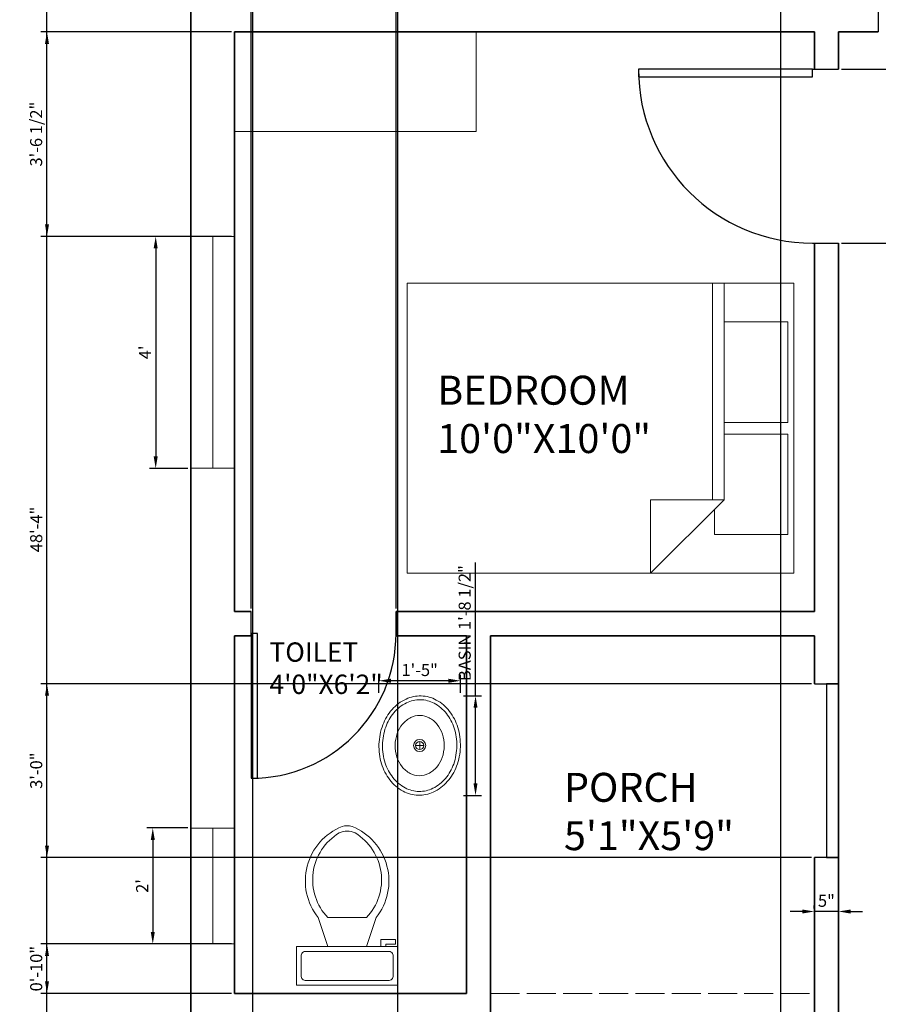
# Model space of a CAD drawing. Units: inches. Extents: x 3889 to 4254, y 3310 to 3958.
# Tile 3 of 6: x 3889 to 4067, y 3534 to 3738. Entities that reach past the tile are written whole.
import ezdxf

# ---------------------------------------------------------------- set-up
doc = ezdxf.new("R2010")
doc.units = ezdxf.units.IN
doc.linetypes.add('ACAD_ISO02W100', pattern=[15, 12, -3])
for name, color, linetype, lineweight in [('A-AREA-IDEN', 11, 'Continuous', 18), ('A-FLOR-FIXT', 130, 'Continuous', 18), ('A-FLOR-OVHD', 7, 'ACAD_ISO02W100', 18), ('A-WALL', 7, 'Continuous', 35), ('DIM', 81, 'Continuous', 18), ('DOOR', 1, 'Continuous', 25), ('FURNITURES', 130, 'Continuous', 18), ('WINDOW', 3, 'Continuous', 18)]:
    doc.layers.add(name, color=color, linetype=linetype, lineweight=lineweight)
doc.styles.get("Standard").update_dxf_attribs({"font": 'arial.ttf'})
doc.dimstyles.new('ISO-25', dxfattribs={"dimtxt": 2.5, "dimasz": 2.5, "dimexe": 1.25, "dimexo": 0.625, "dimtad": 1, "dimlunit": 3, "dimtxsty": 'Standard', "dimcen": 2.5, "dimadec": 0, "dimazin": 0, "dimtfac": 1, "dimtmove": 0, "dimatfit": 3, "dimfxl": 1, "dimarcsym": 0})

# ---------------------------------------------------------------- blocks, each defined once
blk = doc.blocks.new('*U2')
for p, q in [((0, 0), (0, -6)), ((-40, 0), (-40, -6))]:
    blk.add_line(p, q)
blk.add_lwpolyline([(0, 0), (0, 40), (-1.75, 40), (-1.75, 0)], close=True)
blk.add_arc((0, 0), 40, 90, 180)
blk = doc.blocks.new('Bed - Queen')
for p, q in [((0, -80.00003), (0, 0)), ((0, 0), (59.99999, 0)), ((59.99999, 0), (59.99999, -80.00003)), ((7.99999, -1.2), (28.79998, -1.2)), ((7.99999, -14.4), (7.99999, -1.2)), ((28.79998, -1.2), (28.79998, -14.4)), ((31.19999, -1.2), (51.99999, -1.2)), ((31.19999, -14.4), (31.19999, -1.2)), ((51.99999, -1.2), (51.99999, -16.4)), ((0, -14.4), (44.8, -14.4)), ((59.99999, -29.6), (44.8, -14.4)), ((44.8, -14.4), (44.8, -29.6)), ((44.8, -16.8), (0, -16.8)), ((51.99999, -16.4), (46.79936, -16.4)), ((44.8, -29.6), (59.99999, -29.6)), ((59.99999, -80.00003), (0, -80.00003))]:
    blk.add_line(p, q)
blk = doc.blocks.new('Toilet - top')
for p, q in [((9.5, -6), (9.5, -2)), ((-8, -8.5), (-8, -8)), ((-7, -8), (-7, -9.5)), ((-4, -8), (-6, -14)), ((4, -8), (6, -14)), ((-10, -8.5), (-8, -8.5)), ((-10, -9.5), (-10, -8.5)), ((-7, -9.5), (-10, -9.5)), ((4, -14), (-4, -14))]:
    blk.add_line(p, q)
blk.add_lwpolyline([(10.5, -8), (10.5, 0), (-10.5, 0), (-10.5, -8)], close=True)
for points in [[(-9.5, -2), (-9.5, -6)], [(8.5, -1), (-8.5, -1)], [(-8.5, -7), (8.5, -7)]]:
    blk.add_lwpolyline(points)
for centre, radius, start, end in [((-8.62, -1.88), 0.884, 81.8699, 188.1301), ((8.62, -1.88), 0.884, 351.8699, 98.1301), ((-8.62, -6.12), 0.884, 171.8699, 278.1301), ((8.62, -6.12), 0.884, 261.8699, 8.1301), ((3.52, -21.58), 12.17, 141.4691, 247.9714), ((4.2, -21.82), 11.33, 136.3677, 238.9468), ((-3.52, -21.58), 12.17, 292.0284, 38.5307), ((-4.2, -21.82), 11.33, 301.053, 43.6321), ((0, -27.88), 4, 245.7318, 294.2682), ((0, -29), 4, 254.8605, 285.1395)]:
    blk.add_arc(centre, radius, start, end)
blk = doc.blocks.new('Sink - Oval top')
for p, q in [((-1, 0), (1, 0)), ((0, 1), (0, -1))]:
    blk.add_line(p, q)
for points in [[(-12.23, 0.39, 0.117634), (-11.46, -3.36, 0.104469), (-8.88, -6.8, 0.090016), (-5.08, -9.07, 0.08192), (-0.32, -10.02, 0.08192), (4.49, -9.38, 0.090016), (8.42, -7.36, 0.104469), (11.22, -4.09, 0.117634), (12.23, -0.39, 0.117634), (11.46, 3.36, 0.104469), (8.88, 6.8, 0.090016), (5.08, 9.07, 0.08192), (0.32, 10.02, 0.08192), (-4.49, 9.38, 0.090016), (-8.42, 7.36, 0.104469), (-11.22, 4.09, 0.117634)], [(-11.29, 0.16, 0.118622), (-10.52, -3.25, 0.104678), (-8.07, -6.36, 0.089562), (-4.54, -8.37, 0.081185), (-0.13, -9.15, 0.081185), (4.3, -8.49, 0.089562), (7.89, -6.58, 0.104678), (10.42, -3.55, 0.118622), (11.29, -0.16, 0.118622), (10.52, 3.25, 0.104678), (8.07, 6.36, 0.089562), (4.54, 8.37, 0.081185), (0.13, 9.15, 0.081185), (-4.3, 8.49, 0.089562), (-7.89, 6.58, 0.104678), (-10.42, 3.55, 0.118622)], [(-7.42, 0.08, 0.118283), (-6.91, -2.17, 0.104607), (-5.29, -4.21, 0.089718), (-2.97, -5.53, 0.081436), (-0.07, -6.04, 0.081436), (2.84, -5.59, 0.089718), (5.2, -4.33, 0.104607), (6.86, -2.32, 0.118283), (7.42, -0.08, 0.118283), (6.91, 2.17, 0.104607), (5.29, 4.21, 0.089718), (2.97, 5.53, 0.081436), (0.07, 6.04, 0.081436), (-2.84, 5.59, 0.089718), (-5.2, 4.33, 0.104607), (-6.86, 2.32, 0.118283)]]:
    blk.add_lwpolyline(points, format="xyb", close=True)
for radius in [1.5, 1]:
    blk.add_circle((0, 0), radius)
blk = doc.blocks.new('*D22')
at = {"layer": 'Defpoints', "color": 0, "transparency": 16777216}
for p in [(3924.84, 3692.76), (3917.54, 3644.76), (3924.84, 3644.76)]:
    blk.add_point(p, dxfattribs=at)
at = {"layer": 'DIM', "color": 0, "lineweight": -2, "transparency": 16777216}
for p, q in [((3924.22, 3692.76), (3916.29, 3692.76)), ((3917.54, 3690.26), (3917.54, 3647.26)), ((3924.22, 3644.76), (3916.29, 3644.76))]:
    blk.add_line(p, q, dxfattribs=at)
at = {"layer": 'DIM', "color": 0, "transparency": 16777216}
for points in [[(3917.12, 3690.26), (3917.96, 3690.26), (3917.54, 3692.76)], [(3917.12, 3647.26), (3917.96, 3647.26), (3917.54, 3644.76)]]:
    blk.add_solid(points, dxfattribs=at)
at = {"layer": 'DIM', "color": 0, "transparency": 16777216, "insert": (3915.67, 3668.76), "char_height": 2.5, "attachment_point": 5, "rotation": 90}
blk.add_mtext("4'", dxfattribs=at)
blk = doc.blocks.new('*D23')
at = {"layer": 'Defpoints', "color": 0, "transparency": 16777216}
for p in [(3924.84, 3570.33), (3916.94, 3546.33), (3924.84, 3546.33)]:
    blk.add_point(p, dxfattribs=at)
at = {"layer": 'DIM', "color": 0, "lineweight": -2, "transparency": 16777216}
for p, q in [((3924.22, 3570.33), (3915.69, 3570.33)), ((3916.94, 3567.83), (3916.94, 3548.83)), ((3924.22, 3546.33), (3915.69, 3546.33))]:
    blk.add_line(p, q, dxfattribs=at)
at = {"layer": 'DIM', "color": 0, "transparency": 16777216}
for points in [[(3916.52, 3567.83), (3917.36, 3567.83), (3916.94, 3570.33)], [(3916.52, 3548.83), (3917.36, 3548.83), (3916.94, 3546.33)]]:
    blk.add_solid(points, dxfattribs=at)
at = {"layer": 'DIM', "color": 0, "transparency": 16777216, "insert": (3915.06, 3558.33), "char_height": 2.5, "attachment_point": 5, "rotation": 90}
blk.add_mtext("2'", dxfattribs=at)
blk = doc.blocks.new('*D40')
at = {"layer": 'Defpoints', "color": 0, "transparency": 16777216}
for p in [(4053.84, 3553.05), (4053.84, 3553.05), (4058.84, 3553.05)]:
    blk.add_point(p, dxfattribs=at)
at = {"layer": 'DIM', "color": 0, "lineweight": -2, "transparency": 16777216}
for p, q in [((4053.84, 3553.67), (4053.84, 3554.3)), ((4058.84, 3553.67), (4058.84, 3554.3)), ((4051.34, 3553.05), (4048.84, 3553.05)), ((4058.84, 3553.05), (4053.84, 3553.05)), ((4061.34, 3553.05), (4063.84, 3553.05))]:
    blk.add_line(p, q, dxfattribs=at)
at = {"layer": 'DIM', "color": 0, "transparency": 16777216}
for points in [[(4051.34, 3553.46), (4051.34, 3552.63), (4053.84, 3553.05)], [(4061.34, 3553.46), (4061.34, 3552.63), (4058.84, 3553.05)]]:
    blk.add_solid(points, dxfattribs=at)
at = {"layer": 'DIM', "color": 0, "transparency": 16777216, "insert": (4056.34, 3554.94), "char_height": 2.5, "attachment_point": 5}
blk.add_mtext('5"', dxfattribs=at)
blk = doc.blocks.new('WIN-48x9')
blk.add_line((4.5, 48), (4.5, 0))
blk.add_lwpolyline([(0, 48), (9, 48), (9, 0), (0, 0)], close=True)
blk = doc.blocks.new('WIN-24x9')
blk.add_line((24, 4.5), (0, 4.5))
blk.add_lwpolyline([(24, 9), (24, 0), (0, 0), (0, 9)], close=True)
blk = doc.blocks.new('*D49')
at = {"layer": 'Defpoints', "color": 0, "transparency": 16777216}
for p in [(3980.63, 3597.7), (3983.73, 3597.7), (3980.63, 3577.07)]:
    blk.add_point(p, dxfattribs=at)
at = {"layer": 'DIM', "color": 0, "lineweight": -2, "transparency": 16777216}
for p, q in [((3983.73, 3597.7), (3983.73, 3625.26)), ((3981.26, 3597.7), (3984.98, 3597.7)), ((3983.73, 3579.57), (3983.73, 3595.2)), ((3981.26, 3577.07), (3984.98, 3577.07))]:
    blk.add_line(p, q, dxfattribs=at)
at = {"layer": 'DIM', "color": 0, "transparency": 16777216}
for points in [[(3983.31, 3595.2), (3984.14, 3595.2), (3983.73, 3597.7)], [(3983.31, 3579.57), (3984.14, 3579.57), (3983.73, 3577.07)]]:
    blk.add_solid(points, dxfattribs=at)
at = {"layer": 'DIM', "color": 0, "transparency": 16777216, "insert": (3981.81, 3612.73), "char_height": 2.5, "attachment_point": 5, "rotation": 90}
blk.add_mtext('BASIN 1\'-8 1/2"', dxfattribs=at)
blk = doc.blocks.new('*D50')
at = {"layer": 'Defpoints', "color": 0, "transparency": 16777216}
for p in [(3963.71, 3600.8), (3963.71, 3597.7), (3980.63, 3597.7)]:
    blk.add_point(p, dxfattribs=at)
at = {"layer": 'DIM', "color": 0, "lineweight": -2, "transparency": 16777216}
for p, q in [((3963.71, 3598.33), (3963.71, 3602.05)), ((3978.13, 3600.8), (3966.21, 3600.8)), ((3980.63, 3598.33), (3980.63, 3602.05))]:
    blk.add_line(p, q, dxfattribs=at)
at = {"layer": 'DIM', "color": 0, "transparency": 16777216}
for points in [[(3966.21, 3601.22), (3966.21, 3600.38), (3963.71, 3600.8)], [(3978.13, 3601.22), (3978.13, 3600.38), (3980.63, 3600.8)]]:
    blk.add_solid(points, dxfattribs=at)
at = {"layer": 'DIM', "color": 0, "transparency": 16777216, "insert": (3972.17, 3602.7), "char_height": 2.5, "attachment_point": 5}
blk.add_mtext('1\'-5"', dxfattribs=at)
blk = doc.blocks.new('*D73')
at = {"layer": 'Defpoints', "color": 0, "transparency": 16777216}
for p in [(3895.04, 3735.11), (3933.84, 3735.11), (3933.84, 3692.76)]:
    blk.add_point(p, dxfattribs=at)
at = {"layer": 'DIM', "color": 0, "lineweight": -2, "transparency": 16777216}
for p, q in [((3933.22, 3735.11), (3893.79, 3735.11)), ((3895.04, 3695.26), (3895.04, 3732.61)), ((3933.22, 3692.76), (3893.79, 3692.76))]:
    blk.add_line(p, q, dxfattribs=at)
at = {"layer": 'DIM', "color": 0, "transparency": 16777216}
for points in [[(3894.63, 3732.61), (3895.46, 3732.61), (3895.04, 3735.11)], [(3894.63, 3695.26), (3895.46, 3695.26), (3895.04, 3692.76)]]:
    blk.add_solid(points, dxfattribs=at)
at = {"layer": 'DIM', "color": 0, "transparency": 16777216, "insert": (3893.12, 3713.93), "char_height": 2.5, "attachment_point": 5, "rotation": 90}
blk.add_mtext('3\'-6 1/2"', dxfattribs=at)
blk = doc.blocks.new('*D74')
at = {"layer": 'Defpoints', "color": 0, "transparency": 16777216}
for p in [(3895.04, 3546.33), (3933.84, 3546.33), (3933.84, 3536.11)]:
    blk.add_point(p, dxfattribs=at)
at = {"layer": 'DIM', "color": 0, "lineweight": -2, "transparency": 16777216}
for p, q in [((3933.22, 3546.33), (3893.79, 3546.33)), ((3895.04, 3538.61), (3895.04, 3543.83)), ((3933.22, 3536.11), (3893.79, 3536.11))]:
    blk.add_line(p, q, dxfattribs=at)
at = {"layer": 'DIM', "color": 0, "transparency": 16777216}
for points in [[(3894.63, 3543.83), (3895.46, 3543.83), (3895.04, 3546.33)], [(3894.63, 3538.61), (3895.46, 3538.61), (3895.04, 3536.11)]]:
    blk.add_solid(points, dxfattribs=at)
at = {"layer": 'DIM', "color": 0, "transparency": 16777216, "insert": (3893.14, 3541.22), "char_height": 2.5, "attachment_point": 5, "rotation": 90}
blk.add_mtext('0\'-10"', dxfattribs=at)
blk = doc.blocks.new('*D86')
at = {"layer": 'Defpoints', "color": 0, "transparency": 16777216}
for p in [(4046.84, 3865.11), (4110.69, 3865.11), (4110.69, 3312.31)]:
    blk.add_point(p, dxfattribs=at)
at = {"layer": 'DIM', "color": 0, "lineweight": -2, "transparency": 16777216}
for p, q in [((4046.84, 3864.48), (4046.84, 3311.06)), ((4110.69, 3864.48), (4110.69, 3311.06)), ((4049.34, 3312.31), (4108.19, 3312.31))]:
    blk.add_line(p, q, dxfattribs=at)
at = {"layer": 'DIM', "color": 0, "transparency": 16777216}
for points in [[(4049.34, 3312.72), (4049.34, 3311.89), (4046.84, 3312.31)], [(4108.19, 3312.72), (4108.19, 3311.89), (4110.69, 3312.31)]]:
    blk.add_solid(points, dxfattribs=at)
at = {"layer": 'DIM', "color": 0, "transparency": 16777216, "insert": (4078.77, 3314.2), "char_height": 2.5, "attachment_point": 5}
blk.add_mtext('5\'-4"', dxfattribs=at)
blk = doc.blocks.new('*D87')
at = {"layer": 'Defpoints', "color": 0, "transparency": 16777216}
for p in [(4058.84, 3727.38), (4058.84, 3691.38), (4088.64, 3691.38)]:
    blk.add_point(p, dxfattribs=at)
at = {"layer": 'DIM', "color": 0, "lineweight": -2, "transparency": 16777216}
for p, q in [((4059.47, 3727.38), (4089.89, 3727.38)), ((4088.64, 3724.88), (4088.64, 3693.88)), ((4059.47, 3691.38), (4089.89, 3691.38))]:
    blk.add_line(p, q, dxfattribs=at)
at = {"layer": 'DIM', "color": 0, "transparency": 16777216}
for points in [[(4088.23, 3724.88), (4089.06, 3724.88), (4088.64, 3727.38)], [(4088.23, 3693.88), (4089.06, 3693.88), (4088.64, 3691.38)]]:
    blk.add_solid(points, dxfattribs=at)
at = {"layer": 'DIM', "color": 0, "transparency": 16777216, "insert": (4086.74, 3709.38), "char_height": 2.5, "attachment_point": 5, "rotation": 90}
blk.add_mtext('3\'-0"', dxfattribs=at)
blk = doc.blocks.new('*D91')
at = {"layer": 'Defpoints', "color": 0, "transparency": 16777216}
for p in [(3895.04, 3600.19), (4053.84, 3600.19), (4053.84, 3564.19)]:
    blk.add_point(p, dxfattribs=at)
at = {"layer": 'DIM', "color": 0, "lineweight": -2, "transparency": 16777216}
for p, q in [((4053.22, 3600.19), (3893.79, 3600.19)), ((3895.04, 3566.69), (3895.04, 3597.69)), ((4053.22, 3564.19), (3893.79, 3564.19))]:
    blk.add_line(p, q, dxfattribs=at)
at = {"layer": 'DIM', "color": 0, "transparency": 16777216}
for points in [[(3894.63, 3597.69), (3895.46, 3597.69), (3895.04, 3600.19)], [(3894.63, 3566.69), (3895.46, 3566.69), (3895.04, 3564.19)]]:
    blk.add_solid(points, dxfattribs=at)
at = {"layer": 'DIM', "color": 0, "transparency": 16777216, "insert": (3893.14, 3582.19), "char_height": 2.5, "attachment_point": 5, "rotation": 90}
blk.add_mtext('3\'-0"', dxfattribs=at)
blk = doc.blocks.new('*D92')
at = {"layer": 'Defpoints', "color": 0, "transparency": 16777216}
for p in [(3937.55, 3860.11), (3967.55, 3860.11), (3967.55, 3312.31)]:
    blk.add_point(p, dxfattribs=at)
at = {"layer": 'DIM', "color": 0, "lineweight": -2, "transparency": 16777216}
for p, q in [((3937.55, 3859.48), (3937.55, 3311.06)), ((3967.55, 3859.48), (3967.55, 3311.06)), ((3940.05, 3312.31), (3965.05, 3312.31))]:
    blk.add_line(p, q, dxfattribs=at)
at = {"layer": 'DIM', "color": 0, "transparency": 16777216}
for points in [[(3940.05, 3312.72), (3940.05, 3311.89), (3937.55, 3312.31)], [(3965.05, 3312.72), (3965.05, 3311.89), (3967.55, 3312.31)]]:
    blk.add_solid(points, dxfattribs=at)
at = {"layer": 'DIM', "color": 0, "transparency": 16777216, "insert": (3952.55, 3314.21), "char_height": 2.5, "attachment_point": 5}
blk.add_mtext('2\'-6"', dxfattribs=at)
blk = doc.blocks.new('*D93')
at = {"layer": 'Defpoints', "color": 0, "transparency": 16777216}
for p in [(3967.28, 3951.91), (3937.28, 3615.11), (3967.28, 3615.11)]:
    blk.add_point(p, dxfattribs=at)
at = {"layer": 'DIM', "color": 0, "lineweight": -2, "transparency": 16777216}
for p, q in [((3937.28, 3615.73), (3937.28, 3953.16)), ((3967.28, 3615.73), (3967.28, 3953.16)), ((3939.78, 3951.91), (3964.78, 3951.91))]:
    blk.add_line(p, q, dxfattribs=at)
at = {"layer": 'DIM', "color": 0, "transparency": 16777216}
for points in [[(3939.78, 3952.32), (3939.78, 3951.49), (3937.28, 3951.91)], [(3964.78, 3952.32), (3964.78, 3951.49), (3967.28, 3951.91)]]:
    blk.add_solid(points, dxfattribs=at)
at = {"layer": 'DIM', "color": 0, "transparency": 16777216, "insert": (3952.28, 3953.81), "char_height": 2.5, "attachment_point": 5}
blk.add_mtext('2\'-6"', dxfattribs=at)
blk = doc.blocks.new('*D95')
at = {"layer": 'Defpoints', "color": 0, "transparency": 16777216}
for p in [(4046.84, 3865.11), (4098.84, 3860.11), (4098.84, 3312.31)]:
    blk.add_point(p, dxfattribs=at)
at = {"layer": 'DIM', "color": 0, "lineweight": -2, "transparency": 16777216}
for p, q in [((4046.84, 3864.48), (4046.84, 3311.06)), ((4098.84, 3859.48), (4098.84, 3311.06)), ((4049.34, 3312.31), (4096.34, 3312.31))]:
    blk.add_line(p, q, dxfattribs=at)
at = {"layer": 'DIM', "color": 0, "transparency": 16777216}
for points in [[(4049.34, 3312.72), (4049.34, 3311.89), (4046.84, 3312.31)], [(4096.34, 3312.72), (4096.34, 3311.89), (4098.84, 3312.31)]]:
    blk.add_solid(points, dxfattribs=at)
at = {"layer": 'DIM', "color": 0, "transparency": 16777216, "insert": (4072.84, 3314.18), "char_height": 2.5, "attachment_point": 5}
blk.add_mtext('4\'-4"', dxfattribs=at)
blk = doc.blocks.new('*D97')
at = {"layer": 'Defpoints', "color": 0, "transparency": 16777216}
for p in [(3895.04, 3922.11), (3924.84, 3922.11), (3924.84, 3342.11)]:
    blk.add_point(p, dxfattribs=at)
at = {"layer": 'DIM', "color": 0, "lineweight": -2, "transparency": 16777216}
for p, q in [((3924.22, 3922.11), (3893.79, 3922.11)), ((3895.04, 3344.61), (3895.04, 3919.61)), ((3924.22, 3342.11), (3893.79, 3342.11))]:
    blk.add_line(p, q, dxfattribs=at)
at = {"layer": 'DIM', "color": 0, "transparency": 16777216}
for points in [[(3894.63, 3919.61), (3895.46, 3919.61), (3895.04, 3922.11)], [(3894.63, 3344.61), (3895.46, 3344.61), (3895.04, 3342.11)]]:
    blk.add_solid(points, dxfattribs=at)
at = {"layer": 'DIM', "color": 0, "transparency": 16777216, "insert": (3893.14, 3632.11), "char_height": 2.5, "attachment_point": 5, "rotation": 90}
blk.add_mtext('48\'-4"', dxfattribs=at)

msp = doc.modelspace()

# ---------------------------------------------------------------- linework, layer by layer
at = {"layer": 'A-FLOR-OVHD', "ltscale": 0.5}
msp.add_line((3986.843, 3536.107), (4053.843, 3536.107), dxfattribs=at)
at = {"layer": 'A-WALL'}
for p, q in [((3924.843, 3342.107), (3924.843, 3922.107)), ((3933.843, 3735.107), (4053.843, 3735.107)), ((3933.843, 3615.107), (3933.843, 3735.107)), ((4053.843, 3727.381), (4053.843, 3735.107)), ((4058.843, 3727.381), (4058.843, 3735.107)), ((4058.843, 3735.107), (4067.08, 3735.107)), ((4053.843, 3615.107), (4053.843, 3691.381)), ((4058.843, 3610.107), (4058.843, 3691.381)), ((3933.843, 3615.107), (3937.284, 3615.107)), ((3967.284, 3615.107), (4053.843, 3615.107)), ((4058.843, 3511.107), (4058.843, 3615.107)), ((3933.843, 3610.107), (3937.284, 3610.107)), ((3933.843, 3610.107), (3937.284, 3610.107)), ((3933.843, 3536.107), (3933.843, 3610.107)), ((3967.284, 3610.107), (3981.843, 3610.107)), ((3981.843, 3536.107), (3981.843, 3610.107)), ((3986.843, 3531.107), (3986.843, 3610.107)), ((3986.843, 3610.107), (4053.843, 3610.107)), ((4053.843, 3600.193), (4053.843, 3610.107)), ((4053.843, 3531.107), (4053.843, 3564.193)), ((3933.843, 3536.107), (3981.843, 3536.107))]:
    msp.add_line(p, q, dxfattribs=at)
at = {"layer": 'DOOR'}
for points in [[(3937.284, 3610.107), (3937.284, 3615.107)], [(3967.284, 3615.107), (3967.284, 3610.107)], [(4053.843, 3600.193), (4058.843, 3600.193), (4058.843, 3564.193), (4053.843, 3564.193)]]:
    msp.add_lwpolyline(points, dxfattribs=at)
msp.add_lwpolyline([(4058.843, 3600.193), (4056.343, 3600.193), (4056.343, 3564.193), (4058.843, 3564.193)], close=True, dxfattribs=at)
at = {"layer": 'FURNITURES'}
msp.add_lwpolyline([(3933.843, 3735.107), (3983.833, 3735.107), (3983.833, 3714.466), (3933.843, 3714.466)], close=True, dxfattribs=at)

# ---------------------------------------------------------------- block references
at = {"layer": 'A-FLOR-FIXT', "xscale": 0.8405294792783253, "yscale": 0.8405294792783253, "zscale": 0.8405294792783253, "rotation": 90}
msp.add_blockref('Sink - Oval top', (3972.169, 3587.386), dxfattribs=at)
at = {"layer": 'A-FLOR-FIXT', "rotation": 180}
msp.add_blockref('Toilet - top', (3957.155, 3537.784), dxfattribs=at)
at = {"layer": 'DOOR', "xscale": 0.75, "yscale": 0.75, "zscale": 0.75}
msp.add_blockref('*U2', (4097.08, 3739.607), dxfattribs=at)
at = {"layer": 'DOOR'}
for p, xscale, yscale, zscale, rotation in [((4053.443, 3727.381), 0.9, 0.9, 0.9, 90), ((3937.284, 3610.607), 0.75, 0.75, 0.75, 180)]:
    msp.add_blockref('*U2', p, dxfattribs=dict(at, xscale=xscale, yscale=yscale, zscale=zscale, rotation=rotation))
at = {"layer": 'FURNITURES', "rotation": 270}
msp.add_blockref('Bed - Queen', (4049.566, 3683.054), dxfattribs=at)
at = {"layer": 'WINDOW'}
msp.add_blockref('WIN-48x9', (3924.843, 3644.762), dxfattribs=at)
at = {"layer": 'WINDOW', "rotation": 89.9999999999971}
msp.add_blockref('WIN-24x9', (3933.843, 3546.326), dxfattribs=at)

# ---------------------------------------------------------------- texts
at = {"layer": 'A-AREA-IDEN', "attachment_point": 1}
for s, insert, char_height in [('BEDROOM\\P10\'0"X10\'0"', (3975.798, 3663.928), 6), ('TOILET\\P4\'0"X6\'2"', (3941.088, 3608.735), 4), ('PORCH\\P5\'1"X5\'9"', (4002.03, 3581.743), 6)]:
    msp.add_mtext_dynamic_manual_height_columns(s, width=76.4548, gutter_width=12.5, heights=[0], dxfattribs=dict(at, insert=insert, char_height=char_height))

# ---------------------------------------------------------------- dimensions: what is measured, and where the dimension line sits
at = {"layer": 'DIM'}
for base, p1, p2, override, picture, middle in [((3967.284, 3951.907), (3937.284, 3615.107), (3967.284, 3615.107), {"dimdec": 1, "dimlfac": 1, "dimrnd": 0, "dimzin": 1, "dimdsep": 46, "dimlunit": 4, "dimfrac": 2}, '*D93', (3952.284, 3953.808)), ((4110.69, 3312.307), (4046.843, 3865.107), (4110.69, 3865.107), {"dimdec": 1, "dimlfac": 1, "dimrnd": 0, "dimzin": 1, "dimdsep": 46, "dimlunit": 4, "dimfrac": 2}, '*D86', (4078.766, 3314.203)), ((4098.843, 3312.307), (4046.843, 3865.107), (4098.843, 3860.107), {"dimdec": 1, "dimlfac": 1, "dimrnd": 0, "dimzin": 1, "dimdsep": 46, "dimlunit": 4, "dimfrac": 2}, '*D95', (4072.843, 3314.182)), ((3967.546, 3312.307), (3937.546, 3860.107), (3967.546, 3860.107), {"dimdec": 1, "dimlfac": 1, "dimrnd": 0, "dimzin": 1, "dimdsep": 46, "dimlunit": 4, "dimfrac": 2}, '*D92', (3952.546, 3314.208)), ((4053.843, 3553.048), (4058.843, 3553.048), (4053.843, 3553.048), {"dimclrd": 0, "dimclre": 0, "dimclrt": 0}, '*D40', (4056.343, 3554.944))]:
    dim = msp.add_linear_dim(base=base, p1=p1, p2=p2, dimstyle='ISO-25', override=override, dxfattribs=at)
    dim.commit()
    dim.dimension.update_dxf_attribs({"geometry": picture, "text_midpoint": middle})
for base, p1, p2, angle, override, picture, middle in [((3895.043, 3922.107), (3924.843, 3342.107), (3924.843, 3922.107), 90, {"dimdec": 1, "dimlfac": 1, "dimrnd": 0, "dimzin": 1, "dimdsep": 46, "dimlunit": 4, "dimfrac": 2}, '*D97', (3893.141, 3632.107)), ((3895.043, 3735.107), (3933.843, 3692.762), (3933.843, 3735.107), 90, {"dimdec": 1, "dimlfac": 1, "dimrnd": 0, "dimzin": 1, "dimdsep": 46, "dimlunit": 4, "dimfrac": 2}, '*D73', (3893.124, 3713.935)), ((4088.643, 3691.381), (4058.843, 3727.381), (4058.843, 3691.381), 270, {"dimdec": 1, "dimlfac": 1, "dimrnd": 0, "dimzin": 1, "dimdsep": 46, "dimlunit": 4, "dimfrac": 2}, '*D87', (4086.741, 3709.381)), ((3917.54, 3644.762), (3924.843, 3692.762), (3924.843, 3644.762), 90, {"dimclrd": 0, "dimclre": 0, "dimclrt": 0}, '*D22', (3915.665, 3668.762)), ((3963.707, 3600.799), (3980.632, 3597.704), (3963.707, 3597.704), 180, {"dimdec": 1, "dimlfac": 1, "dimrnd": 0, "dimzin": 1, "dimdsep": 46, "dimlunit": 4, "dimfrac": 2}, '*D50', (3972.169, 3602.7)), ((3895.043, 3600.193), (4053.843, 3564.193), (4053.843, 3600.193), 90, {"dimdec": 1, "dimlfac": 1, "dimrnd": 0, "dimzin": 1, "dimdsep": 46, "dimlunit": 4, "dimfrac": 2}, '*D91', (3893.141, 3582.193)), ((3916.941, 3546.326), (3924.843, 3570.326), (3924.843, 3546.326), 90, {"dimclrd": 0, "dimclre": 0, "dimclrt": 0}, '*D23', (3915.061, 3558.326)), ((3895.043, 3546.326), (3933.843, 3536.107), (3933.843, 3546.326), 90, {"dimdec": 1, "dimlfac": 1, "dimrnd": 0, "dimzin": 1, "dimdsep": 46, "dimlunit": 4, "dimfrac": 2}, '*D74', (3893.141, 3541.216))]:
    dim = msp.add_linear_dim(base=base, p1=p1, p2=p2, angle=angle, dimstyle='ISO-25', override=override, dxfattribs=at)
    dim.commit()
    dim.dimension.update_dxf_attribs({"geometry": picture, "text_midpoint": middle})
dim = msp.add_linear_dim(base=(3983.727, 3597.704), p1=(3980.632, 3577.068), p2=(3980.632, 3597.704), angle=90, text='BASIN <>', dimstyle='ISO-25', override={"dimdec": 1, "dimlfac": 1, "dimrnd": 0, "dimzin": 1, "dimdsep": 46, "dimlunit": 4, "dimfrac": 2}, dxfattribs=at)
dim.commit()
dim.dimension.update_dxf_attribs({"geometry": '*D49', "text_midpoint": (3981.81, 3612.734)})

doc.saveas('drawing.dxf')
